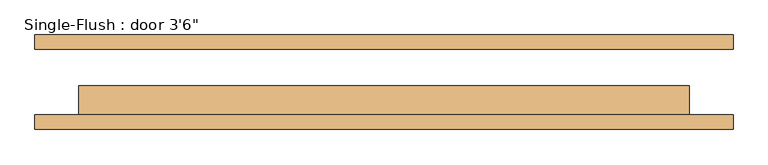
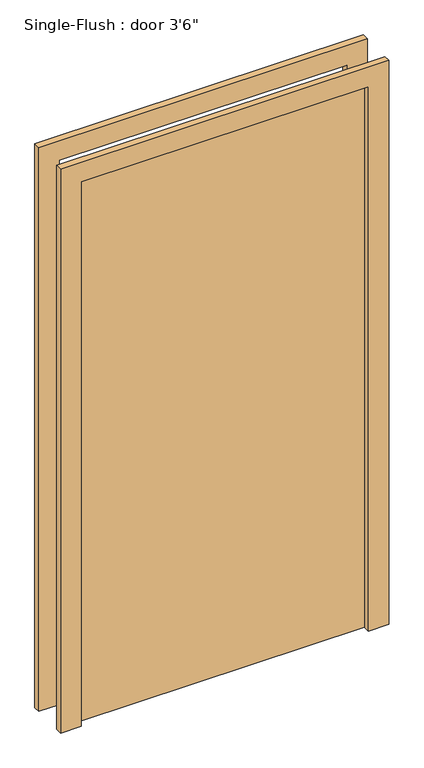
"""IFC4 building model written with IfcOpenShell, lengths in millimetres: door geometry."""

from ifc_helpers import new_model, si_unit, frame, origin, origin_with_axes, place, context, project, spatial, polyline, outline, extrude, source, transform, mapped, element, save


def door_e6ebe4aa(model_context):
    return source(origin(), model_context, "Body", "SweptSolid", [
        extrude(outline(polyline([(2209.8, -609.6), (0.0, -609.6), (0.0, -533.4), (2133.6, -533.4), (2133.6, 533.4), (0.0, 533.4), (0.0, 609.6), (2209.8, 609.6), (2209.8, -609.6)])), frame((0.0, -82.55, 0.0), z_axis=(0.0, 1.0, 0.0), x_axis=(0.0, 0.0, 1.0)), (0.0, 0.0, 1.0), 25.4),
        extrude(outline(polyline([(2209.8, 609.6), (2209.8, -609.6), (0.0, -609.6), (0.0, -533.4), (2133.6, -533.4), (2133.6, 533.4), (0.0, 533.4), (0.0, 609.6), (2209.8, 609.6)])), frame((0.0, 57.15, 0.0), z_axis=(0.0, 1.0, 0.0), x_axis=(0.0, 0.0, 1.0)), (0.0, 0.0, 1.0), 25.4),
        extrude(outline(polyline([(533.4, -6.35), (533.4, -57.15), (-533.4, -57.15), (-533.4, -6.35), (533.4, -6.35)])), origin_with_axes(), (0.0, 0.0, 1.0), 2133.6),
    ])


if __name__ == "__main__":
    model = new_model("IFC4")
    model_context = context("Model", 3, world=origin())
    ifc_project = project(units=[si_unit("LENGTHUNIT", "METRE", prefix="MILLI")], contexts=[model_context])
    site = spatial("IfcSite", under=ifc_project)
    building = spatial("IfcBuilding", under=site)
    placement = place(None, origin())
    door_shape = door_e6ebe4aa(model_context)
    element("IfcDoor", 1, ObjectType="Single-Flush : door 3'6\"", at=placement, inside=building, context=model_context, shape_type="MappedRepresentation", body=[
        mapped(door_shape, transform((0.0, 0.0, 0.0), x_axis=(1.0, 0.0, 0.0), y_axis=(0.0, 1.0, 0.0), z_axis=(0.0, 0.0, 1.0))),
    ])
    save(model, "model.ifc")

# Revit data of these elements
# Type "Single-Flush : door 3'6\""
#   Type Mark = "9"
#   Construction Type Id = "MDOOR"
#   Assembly Code = "C1020"
#   Analytic Construction = "Metal"
#   Thickness = 0' - 2"
#   Heat Transfer Coefficient (U) = 0.651978 BTU/(h·ft²·°F)
#   Height = 7' - 0"
#   Trim Projection Ext = 0' - 1"
#   Trim Projection Int = 0' - 1"
#   Trim Width = 0' - 3"
#   Width = 3' - 6"
#   Define Thermal Properties by = 1
#   Door Material = Door - Panel
#   Frame Material = Door - Frame
#   Visual Light Transmittance = 0
#   Solar Heat Gain Coefficient = 0
#   Function = (empty or 0)
#   Wall Closure = (empty or 0)
# Element 1 (IfcDoor, "Single-Flush : door 3'6\"")
#   Materials on its faces: "Door - Frame", "Door - Panel"
# Materials
#   "Door - Panel": class "Wood", colour RGB 210 159 95, transparency 0, Cost = 0
#   "Door - Frame": colour RGB 118 70 51, transparency 0, Cost = 0
